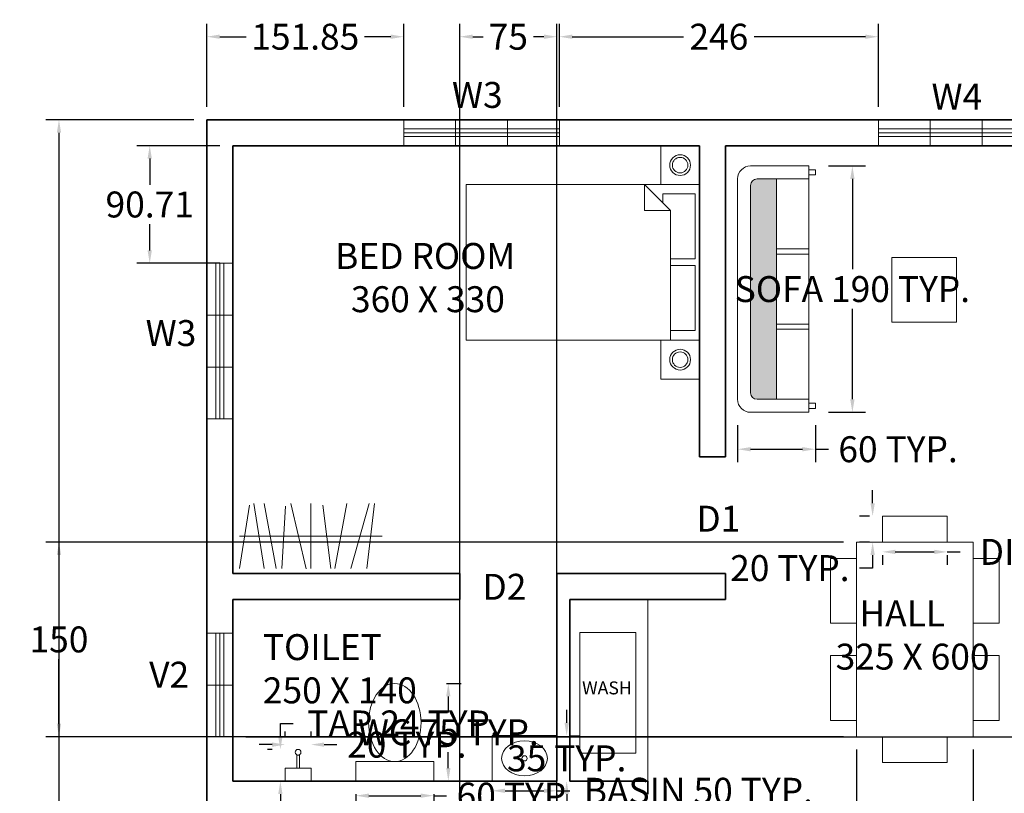
# Model space of a CAD drawing. Units: centimetres. Extents: x 543 to 2148, y 348 to 1642.
# Tile 2 of 4: x 543 to 1302, y 1046 to 1642. Entities that reach past the tile are written whole.
import ezdxf

# ---------------------------------------------------------------- set-up
doc = ezdxf.new("R2010")
doc.units = ezdxf.units.CM
doc.header["$MEASUREMENT"] = 0
for name, color, linetype, lineweight in [('A-ANNO-DIMS', 2, 'Continuous', 18), ('A-ANNO-TEXT', 7, 'Continuous', 18), ('A-AREA-IDEN', 7, 'Continuous', 25), ('A-FLOR-CASE', 8, 'Continuous', 20), ('A-FLOR-FIXT', 8, 'Continuous', 18), ('A-FURN', 8, 'Continuous', 18), ('A-FURN-PATT', 252, 'Continuous', 13), ('A-GLAZ', 4, 'Continuous', 18), ('A-WALL', 7, 'Continuous', 35)]:
    doc.layers.add(name, color=color, linetype=linetype, lineweight=lineweight)
doc.styles.get("Standard").update_dxf_attribs({"font": 'arial.ttf'})
doc.dimstyles.get("Standard").update_dxf_attribs({"dimtxt": 20, "dimasz": 10, "dimexe": 10, "dimexo": 10, "dimgap": 5, "dimtad": 0, "dimtih": 1, "dimtoh": 1, "dimdec": 0, "dimzin": 0, "dimdsep": 46, "dimtxsty": 'Standard', "dimcen": 5, "dimadec": 0, "dimazin": 0, "dimtfac": 1, "dimtdec": 0, "dimtofl": 0, "dimtmove": 0, "dimatfit": 3, "dimfxl": 1, "dimtolj": 1, "dimtzin": 0, "dimarcsym": 0})

# ---------------------------------------------------------------- blocks, each defined once
blk = doc.blocks.new('BED-DOUBLE')
for p, q in [((42.36, 150), (22.36, 130)), ((42.36, 130), (42.36, 150)), ((22.36, 130), (22.36, 30)), ((22.36, 130), (42.36, 130)), ((3.32, 102.87), (3.32, 92.87)), ((3.32, 92.87), (22.36, 92.87)), ((3.32, 77.49), (3.32, 87.49)), ((3.32, 87.49), (22.36, 87.49))]:
    blk.add_line(p, q)
for points in [[(0, 150), (30, 150), (30, 180), (0, 180)], [(180, 150), (180, 30), (0, 30), (0, 150)], [(0, 0), (30, 0), (30, 30), (0, 30)]]:
    blk.add_lwpolyline(points, close=True)
for points in [[(3.32, 102.87), (3.32, 142.87), (28.32, 142.87), (28.32, 135.96)], [(22.36, 37.49), (3.32, 37.49), (3.32, 77.49)]]:
    blk.add_lwpolyline(points)
for centre, radius in [((15, 165), 8), ((15, 165), 6), ((15, 15), 8), ((15, 15), 6)]:
    blk.add_circle(centre, radius)
blk = doc.blocks.new('SOFA-3SEAT')
for p, q in [((10, 190), (55, 190)), ((55, 190), (55, 125.56)), ((55, 190), (55, 187)), ((55, 187), (60, 187)), ((60, 183), (55, 183)), ((60, 187), (60, 183)), ((0, 125.56), (0, 180)), ((10, 125.56), (10, 175)), ((15, 180), (55, 180)), ((30, 125.56), (30, 180)), ((0, 10), (0, 125.56)), ((10, 15), (10, 125.56)), ((55, 126), (30, 126)), ((30, 10), (30, 125.56)), ((55, 122), (30, 122)), ((55, 125.56), (55, 0)), ((55, 68), (30, 68)), ((55, 64), (30, 64)), ((55, 10), (15, 10)), ((55, 0), (10, 0)), ((60, 7), (55, 7)), ((55, 0), (55, 3)), ((55, 3), (60, 3)), ((60, 3), (60, 7))]:
    blk.add_line(p, q)
for centre, radius, start, end in [((10, 180), 10, 90, 180), ((15, 175), 5, 90, 180), ((10, 10), 10, 180, 270), ((15, 15), 5, 180, 270)]:
    blk.add_arc(centre, radius, start, end)
blk = doc.blocks.new('WARDROBE-RAIL')
for p, q in [((0, 0.31), (7.78, 49.18)), ((11.01, 50.31), (19.09, 0.31)), ((19.09, 50.31), (28.16, 0.3)), ((32.55, 0.31), (35.53, 48.25)), ((39.55, 50.31), (51.34, 0)), ((55, 0.31), (55, 50.31)), ((64.34, 49.01), (70.51, 0.27)), ((73.48, 0.31), (82.64, 50.31)), ((99.87, 50.31), (85.87, 0.31)), ((98.25, 0.31), (103.96, 50.31)), ((0, 25.31), (110, 25.31))]:
    blk.add_line(p, q)
blk = doc.blocks.new('WIN-1200')
for p, q in [((40, 20), (40, 0)), ((80, 20), (80, 0)), ((0, 13), (120, 13)), ((0, 10), (120, 10)), ((0, 7), (120, 7))]:
    blk.add_line(p, q)
blk.add_lwpolyline([(0, 20), (120, 20), (120, 0), (0, 0)], close=True)
blk = doc.blocks.new('VENT-800')
for p, q in [((7, 80), (7, 0)), ((10, 80), (10, 0)), ((13, 80), (13, 0)), ((20, 40), (0, 40)), ((20, 0), (0, 0))]:
    blk.add_line(p, q)
blk.add_lwpolyline([(0, 0), (0, 80), (20, 80), (20, 0)])
blk = doc.blocks.new('WC')
blk.add_lwpolyline([(60, 0), (0, 0), (0, 15), (60, 15)], close=True)
blk.add_ellipse((30, 45.11), major_axis=(0, 30.11), ratio=0.671585)
blk = doc.blocks.new('WASHBASIN')
blk.add_lwpolyline([(50, 0), (0, 0), (0, 35), (50, 35)], close=True)
blk.add_circle((25, 17.5), 2)
blk.add_ellipse((25, 17.5), major_axis=(17.65, 0), ratio=0.767259)
blk = doc.blocks.new('WALL-TAP')
for p, q in [((9, 10), (9, 20)), ((9, 20), (11, 20)), ((11, 10), (11, 20))]:
    blk.add_line(p, q)
blk.add_lwpolyline([(0, 0), (20, 0), (20, 10), (0, 10)], close=True)
blk.add_circle((10, 22.21), 2.21)
blk = doc.blocks.new('CHAIR-DINING')
blk.add_lwpolyline([(0, 50), (0, 0), (20, 0), (20, 50)], close=True)
blk = doc.blocks.new('TABLE-SIDE')
blk.add_lwpolyline([(0, 50), (50, 50), (50, 0), (0, 0)], close=True)
blk = doc.blocks.new('*D15')
at = {"layer": 'A-ANNO-DIMS', "color": 0, "lineweight": -2, "transparency": 16777216}
for p, q in [((1218.09, 1231.81), (1248.09, 1231.81)), ((1258.09, 1231.81), (1268.09, 1231.81)), ((1208.09, 1229.31), (1208.09, 1221.81)), ((1258.09, 1229.31), (1258.09, 1221.81))]:
    blk.add_line(p, q, dxfattribs=at)
at = {"layer": 'A-ANNO-DIMS', "color": 0, "transparency": 16777216}
for points in [[(1218.09, 1233.48), (1218.09, 1230.15), (1208.09, 1231.81)], [(1248.09, 1233.48), (1248.09, 1230.15), (1258.09, 1231.81)]]:
    blk.add_solid(points, dxfattribs=at)
at = {"layer": 'Defpoints', "color": 0, "transparency": 16777216}
for p in [(1208.09, 1239.31), (1258.09, 1239.31), (1258.09, 1231.81)]:
    blk.add_point(p, dxfattribs=at)
at = {"layer": 'A-ANNO-DIMS', "color": 0, "transparency": 16777216, "insert": (1421.4, 1231.81), "char_height": 20, "attachment_point": 5}
blk.add_mtext('\\A1;DINING CHAIR 50 TYP.', dxfattribs=at)
blk = doc.blocks.new('*D16')
at = {"layer": 'A-ANNO-DIMS', "color": 0, "lineweight": -2, "transparency": 16777216}
for p, q in [((1200.59, 1269.31), (1200.59, 1279.31)), ((1198.09, 1259.31), (1190.59, 1259.31)), ((1198.09, 1239.31), (1190.59, 1239.31)), ((1200.59, 1229.31), (1200.59, 1219.31)), ((1200.59, 1219.31), (1190.59, 1219.31))]:
    blk.add_line(p, q, dxfattribs=at)
at = {"layer": 'A-ANNO-DIMS', "color": 0, "transparency": 16777216}
for points in [[(1198.93, 1269.31), (1202.26, 1269.31), (1200.59, 1259.31)], [(1198.93, 1229.31), (1202.26, 1229.31), (1200.59, 1239.31)]]:
    blk.add_solid(points, dxfattribs=at)
at = {"layer": 'Defpoints', "color": 0, "transparency": 16777216}
for p in [(1208.09, 1259.31), (1200.59, 1239.31), (1208.09, 1239.31)]:
    blk.add_point(p, dxfattribs=at)
at = {"layer": 'A-ANNO-DIMS', "color": 0, "transparency": 16777216, "insert": (1136.75, 1219.31), "char_height": 20, "attachment_point": 5}
blk.add_mtext('\\A1;20 TYP.', dxfattribs=at)
blk = doc.blocks.new('*D23')
at = {"layer": 'A-ANNO-DIMS', "color": 0, "lineweight": -2, "transparency": 16777216}
for p, q in [((1166.48, 1529.5), (1194.98, 1529.5)), ((1184.98, 1519.5), (1184.98, 1449.85)), ((1184.98, 1349.5), (1184.98, 1419.16)), ((1166.48, 1339.5), (1194.98, 1339.5))]:
    blk.add_line(p, q, dxfattribs=at)
at = {"layer": 'A-ANNO-DIMS', "color": 0, "transparency": 16777216}
for points in [[(1183.31, 1519.5), (1186.65, 1519.5), (1184.98, 1529.5)], [(1183.31, 1349.5), (1186.65, 1349.5), (1184.98, 1339.5)]]:
    blk.add_solid(points, dxfattribs=at)
at = {"layer": 'Defpoints', "color": 0, "transparency": 16777216}
for p in [(1156.48, 1529.5), (1184.98, 1529.5), (1156.48, 1339.5)]:
    blk.add_point(p, dxfattribs=at)
at = {"layer": 'A-ANNO-DIMS', "color": 0, "transparency": 16777216, "insert": (1184.98, 1434.5), "char_height": 20, "attachment_point": 5}
blk.add_mtext('\\A1;SOFA 190 TYP.', dxfattribs=at)
blk = doc.blocks.new('*D24')
at = {"layer": 'A-ANNO-DIMS', "color": 0, "lineweight": -2, "transparency": 16777216}
for p, q in [((1096.48, 1329.5), (1096.48, 1301)), ((1156.48, 1329.5), (1156.48, 1301)), ((1106.48, 1311), (1146.48, 1311)), ((1156.48, 1311), (1166.48, 1311))]:
    blk.add_line(p, q, dxfattribs=at)
at = {"layer": 'A-ANNO-DIMS', "color": 0, "transparency": 16777216}
for points in [[(1106.48, 1312.67), (1106.48, 1309.34), (1096.48, 1311)], [(1146.48, 1312.67), (1146.48, 1309.34), (1156.48, 1311)]]:
    blk.add_solid(points, dxfattribs=at)
at = {"layer": 'Defpoints', "color": 0, "transparency": 16777216}
for p in [(1096.48, 1339.5), (1156.48, 1339.5), (1156.48, 1311)]:
    blk.add_point(p, dxfattribs=at)
at = {"layer": 'A-ANNO-DIMS', "color": 0, "transparency": 16777216, "insert": (1220.21, 1311), "char_height": 20, "attachment_point": 5}
blk.add_mtext('\\A1;60 TYP.', dxfattribs=at)
blk = doc.blocks.new('*D29')
at = {"layer": 'A-ANNO-DIMS', "color": 0, "lineweight": -2, "transparency": 16777216}
for p, q in [((872.08, 1130.32), (883.37, 1130.32)), ((873.37, 1120.32), (873.37, 1108.05)), ((873.37, 1065.09), (873.37, 1077.36)), ((872.08, 1055.09), (883.37, 1055.09))]:
    blk.add_line(p, q, dxfattribs=at)
at = {"layer": 'A-ANNO-DIMS', "color": 0, "transparency": 16777216}
for points in [[(871.7, 1120.32), (875.03, 1120.32), (873.37, 1130.32)], [(871.7, 1065.09), (875.03, 1065.09), (873.37, 1055.09)]]:
    blk.add_solid(points, dxfattribs=at)
at = {"layer": 'Defpoints', "color": 0, "transparency": 16777216}
for p in [(862.08, 1130.32), (873.37, 1130.32), (862.08, 1055.09)]:
    blk.add_point(p, dxfattribs=at)
at = {"layer": 'A-ANNO-DIMS', "color": 0, "transparency": 16777216, "insert": (873.37, 1092.7), "char_height": 20, "attachment_point": 5}
blk.add_mtext('\\A1;WC 75 TYP.', dxfattribs=at)
blk = doc.blocks.new('*D30')
at = {"layer": 'A-ANNO-DIMS', "color": 0, "lineweight": -2, "transparency": 16777216}
for p, q in [((802.08, 1045.09), (802.08, 1033.81)), ((812.08, 1043.81), (852.08, 1043.81)), ((862.08, 1045.09), (862.08, 1033.81)), ((862.08, 1043.81), (872.08, 1043.81))]:
    blk.add_line(p, q, dxfattribs=at)
at = {"layer": 'A-ANNO-DIMS', "color": 0, "transparency": 16777216}
for points in [[(812.08, 1045.47), (812.08, 1042.14), (802.08, 1043.81)], [(852.08, 1045.47), (852.08, 1042.14), (862.08, 1043.81)]]:
    blk.add_solid(points, dxfattribs=at)
at = {"layer": 'Defpoints', "color": 0, "transparency": 16777216}
for p in [(802.08, 1055.09), (862.08, 1055.09), (862.08, 1043.81)]:
    blk.add_point(p, dxfattribs=at)
at = {"layer": 'A-ANNO-DIMS', "color": 0, "transparency": 16777216, "insert": (925.81, 1043.81), "char_height": 20, "attachment_point": 5}
blk.add_mtext('\\A1;60 TYP.', dxfattribs=at)
blk = doc.blocks.new('*D31')
at = {"layer": 'A-ANNO-DIMS', "color": 0, "lineweight": -2, "transparency": 16777216}
for p, q in [((907.14, 1045.09), (907.14, 1037.59)), ((917.14, 1047.59), (947.14, 1047.59)), ((957.14, 1047.59), (967.14, 1047.59)), ((957.14, 1045.09), (957.14, 1037.59))]:
    blk.add_line(p, q, dxfattribs=at)
at = {"layer": 'A-ANNO-DIMS', "color": 0, "transparency": 16777216}
for points in [[(917.14, 1049.26), (917.14, 1045.93), (907.14, 1047.59)], [(947.14, 1049.26), (947.14, 1045.93), (957.14, 1047.59)]]:
    blk.add_solid(points, dxfattribs=at)
at = {"layer": 'Defpoints', "color": 0, "transparency": 16777216}
for p in [(907.14, 1055.09), (957.14, 1055.09), (957.14, 1047.59)]:
    blk.add_point(p, dxfattribs=at)
at = {"layer": 'A-ANNO-DIMS', "color": 0, "transparency": 16777216, "insert": (1066.18, 1047.59), "char_height": 20, "attachment_point": 5}
blk.add_mtext('\\A1;BASIN 50 TYP.', dxfattribs=at)
blk = doc.blocks.new('*D32')
at = {"layer": 'A-ANNO-DIMS', "color": 0, "lineweight": -2, "transparency": 16777216}
for p, q in [((964.64, 1100.09), (964.64, 1110.09)), ((967.14, 1090.09), (974.64, 1090.09)), ((967.14, 1055.09), (974.64, 1055.09)), ((964.64, 1045.09), (964.64, 1035.09))]:
    blk.add_line(p, q, dxfattribs=at)
at = {"layer": 'A-ANNO-DIMS', "color": 0, "transparency": 16777216}
for points in [[(962.97, 1100.09), (966.31, 1100.09), (964.64, 1090.09)], [(962.97, 1045.09), (966.31, 1045.09), (964.64, 1055.09)]]:
    blk.add_solid(points, dxfattribs=at)
at = {"layer": 'Defpoints', "color": 0, "transparency": 16777216}
for p in [(957.14, 1090.09), (964.64, 1090.09), (957.14, 1055.09)]:
    blk.add_point(p, dxfattribs=at)
at = {"layer": 'A-ANNO-DIMS', "color": 0, "transparency": 16777216, "insert": (964.64, 1072.59), "char_height": 20, "attachment_point": 5}
blk.add_mtext('\\A1;35 TYP.', dxfattribs=at)
blk = doc.blocks.new('*D33')
at = {"layer": 'A-ANNO-DIMS', "color": 0, "lineweight": -2, "transparency": 16777216}
for p, q in [((743.83, 1089.51), (743.83, 1099.51)), ((743.83, 1099.51), (753.83, 1099.51)), ((737.5, 1079.51), (733.83, 1079.51)), ((737.5, 1055.09), (733.83, 1055.09)), ((743.83, 1045.09), (743.83, 1035.09))]:
    blk.add_line(p, q, dxfattribs=at)
at = {"layer": 'A-ANNO-DIMS', "color": 0, "transparency": 16777216}
for points in [[(742.17, 1089.51), (745.5, 1089.51), (743.83, 1079.51)], [(742.17, 1045.09), (745.5, 1045.09), (743.83, 1055.09)]]:
    blk.add_solid(points, dxfattribs=at)
at = {"layer": 'Defpoints', "color": 0, "transparency": 16777216}
for p in [(743.83, 1079.51), (747.5, 1079.51), (747.5, 1055.09)]:
    blk.add_point(p, dxfattribs=at)
at = {"layer": 'A-ANNO-DIMS', "color": 0, "transparency": 16777216, "insert": (838.81, 1099.51), "char_height": 20, "attachment_point": 5}
blk.add_mtext('\\A1;TAP 24 TYP.', dxfattribs=at)
blk = doc.blocks.new('*D34')
at = {"layer": 'A-ANNO-DIMS', "color": 0, "lineweight": -2, "transparency": 16777216}
for p, q in [((747.5, 1089.51), (747.5, 1093.18)), ((767.5, 1089.51), (767.5, 1093.18)), ((737.5, 1083.18), (727.5, 1083.18)), ((777.5, 1083.18), (787.5, 1083.18))]:
    blk.add_line(p, q, dxfattribs=at)
at = {"layer": 'A-ANNO-DIMS', "color": 0, "transparency": 16777216}
for points in [[(737.5, 1084.84), (737.5, 1081.51), (747.5, 1083.18)], [(777.5, 1084.84), (777.5, 1081.51), (767.5, 1083.18)]]:
    blk.add_solid(points, dxfattribs=at)
at = {"layer": 'Defpoints', "color": 0, "transparency": 16777216}
for p in [(747.5, 1079.51), (767.5, 1083.18), (767.5, 1079.51)]:
    blk.add_point(p, dxfattribs=at)
at = {"layer": 'A-ANNO-DIMS', "color": 0, "transparency": 16777216, "insert": (841.34, 1083.18), "char_height": 20, "attachment_point": 5}
blk.add_mtext('\\A1;20 TYP.', dxfattribs=at)
blk = doc.blocks.new('*D44')
at = {"layer": 'A-ANNO-DIMS', "color": 0, "lineweight": -2, "transparency": 16777216}
for p, q in [((882.14, 895.09), (882.14, 1639.14)), ((957.14, 895.09), (957.14, 1639.14)), ((892.14, 1629.14), (900.32, 1629.14)), ((947.14, 1629.14), (938.96, 1629.14))]:
    blk.add_line(p, q, dxfattribs=at)
at = {"layer": 'A-ANNO-DIMS', "color": 0, "transparency": 16777216}
for points in [[(892.14, 1630.81), (892.14, 1627.48), (882.14, 1629.14)], [(947.14, 1630.81), (947.14, 1627.48), (957.14, 1629.14)]]:
    blk.add_solid(points, dxfattribs=at)
at = {"layer": 'Defpoints', "color": 0, "transparency": 16777216}
for p in [(957.14, 1629.14), (882.14, 885.09), (957.14, 885.09)]:
    blk.add_point(p, dxfattribs=at)
at = {"layer": 'A-ANNO-DIMS', "color": 0, "transparency": 16777216, "insert": (919.64, 1629.14), "char_height": 20, "attachment_point": 5}
blk.add_mtext('\\A1;75', dxfattribs=at)
blk = doc.blocks.new('*D48')
at = {"layer": 'A-ANNO-DIMS', "color": 0, "lineweight": -2, "transparency": 16777216}
for p, q in [((687.14, 1575.09), (687.14, 1639.14)), ((838.99, 1575.09), (838.99, 1639.14)), ((697.14, 1629.14), (717.42, 1629.14)), ((828.99, 1629.14), (808.71, 1629.14))]:
    blk.add_line(p, q, dxfattribs=at)
at = {"layer": 'A-ANNO-DIMS', "color": 0, "transparency": 16777216}
for points in [[(697.14, 1630.81), (697.14, 1627.48), (687.14, 1629.14)], [(828.99, 1630.81), (828.99, 1627.48), (838.99, 1629.14)]]:
    blk.add_solid(points, dxfattribs=at)
at = {"layer": 'Defpoints', "color": 0, "transparency": 16777216}
for p in [(838.99, 1629.14), (687.14, 1565.09), (838.99, 1565.09)]:
    blk.add_point(p, dxfattribs=at)
at = {"layer": 'A-ANNO-DIMS', "color": 0, "transparency": 16777216, "insert": (763.06, 1629.14), "char_height": 20, "attachment_point": 5}
blk.add_mtext('\\A1;151.85', dxfattribs=at)
blk = doc.blocks.new('*D49')
at = {"layer": 'A-ANNO-DIMS', "color": 0, "lineweight": -2, "transparency": 16777216}
for p, q in [((958.99, 1575.09), (958.99, 1639.14)), ((1205.01, 1575.09), (1205.01, 1639.14)), ((968.99, 1629.14), (1054.74, 1629.14)), ((1195.01, 1629.14), (1109.25, 1629.14))]:
    blk.add_line(p, q, dxfattribs=at)
at = {"layer": 'A-ANNO-DIMS', "color": 0, "transparency": 16777216}
for points in [[(968.99, 1630.81), (968.99, 1627.48), (958.99, 1629.14)], [(1195.01, 1630.81), (1195.01, 1627.48), (1205.01, 1629.14)]]:
    blk.add_solid(points, dxfattribs=at)
at = {"layer": 'Defpoints', "color": 0, "transparency": 16777216}
for p in [(1205.01, 1629.14), (958.99, 1565.09), (1205.01, 1565.09)]:
    blk.add_point(p, dxfattribs=at)
at = {"layer": 'A-ANNO-DIMS', "color": 0, "transparency": 16777216, "insert": (1082, 1629.14), "char_height": 20, "attachment_point": 5}
blk.add_mtext('\\A1;246', dxfattribs=at)
blk = doc.blocks.new('*D59')
at = {"layer": 'A-ANNO-DIMS', "color": 0, "lineweight": -2, "transparency": 16777216}
for p, q in [((717.14, 1089.08), (1916.19, 1089.08)), ((1906.19, 1079.08), (1906.19, 1065.14)), ((1906.19, 1020.76), (1906.19, 1034.7)), ((717.14, 1010.76), (1916.19, 1010.76))]:
    blk.add_line(p, q, dxfattribs=at)
at = {"layer": 'A-ANNO-DIMS', "color": 0, "transparency": 16777216}
for points in [[(1904.52, 1079.08), (1907.86, 1079.08), (1906.19, 1089.08)], [(1904.52, 1020.76), (1907.86, 1020.76), (1906.19, 1010.76)]]:
    blk.add_solid(points, dxfattribs=at)
at = {"layer": 'Defpoints', "color": 0, "transparency": 16777216}
for p in [(707.14, 1089.08), (1906.19, 1089.08), (707.14, 1010.76)]:
    blk.add_point(p, dxfattribs=at)
at = {"layer": 'A-ANNO-DIMS', "color": 0, "transparency": 16777216, "insert": (1906.19, 1049.92), "char_height": 20, "attachment_point": 5}
blk.add_mtext('\\A1;78.33', dxfattribs=at)
blk = doc.blocks.new('*D60')
at = {"layer": 'A-ANNO-DIMS', "color": 0, "lineweight": -2, "transparency": 16777216}
for p, q in [((697.14, 1545.09), (633.09, 1545.09)), ((643.09, 1535.09), (643.09, 1514.95)), ((643.09, 1464.38), (643.09, 1484.52)), ((697.14, 1454.38), (633.09, 1454.38))]:
    blk.add_line(p, q, dxfattribs=at)
at = {"layer": 'A-ANNO-DIMS', "color": 0, "transparency": 16777216}
for points in [[(641.42, 1535.09), (644.76, 1535.09), (643.09, 1545.09)], [(641.42, 1464.38), (644.76, 1464.38), (643.09, 1454.38)]]:
    blk.add_solid(points, dxfattribs=at)
at = {"layer": 'Defpoints', "color": 0, "transparency": 16777216}
for p in [(643.09, 1545.09), (707.14, 1545.09), (707.14, 1454.38)]:
    blk.add_point(p, dxfattribs=at)
at = {"layer": 'A-ANNO-DIMS', "color": 0, "transparency": 16777216, "insert": (643.09, 1499.74), "char_height": 20, "attachment_point": 5}
blk.add_mtext('\\A1;90.71', dxfattribs=at)
blk = doc.blocks.new('*D64')
at = {"layer": 'A-ANNO-DIMS', "color": 0, "lineweight": -2, "transparency": 16777216}
for p, q in [((1188.09, 1079.31), (1188.09, 351.04)), ((1278.09, 1079.31), (1278.09, 351.04)), ((1198.09, 361.04), (1213.8, 361.04)), ((1268.09, 361.04), (1252.38, 361.04))]:
    blk.add_line(p, q, dxfattribs=at)
at = {"layer": 'A-ANNO-DIMS', "color": 0, "transparency": 16777216}
for points in [[(1198.09, 362.71), (1198.09, 359.38), (1188.09, 361.04)], [(1268.09, 362.71), (1268.09, 359.38), (1278.09, 361.04)]]:
    blk.add_solid(points, dxfattribs=at)
at = {"layer": 'Defpoints', "color": 0, "transparency": 16777216}
for p in [(1188.09, 1089.31), (1278.09, 1089.31), (1278.09, 361.04)]:
    blk.add_point(p, dxfattribs=at)
at = {"layer": 'A-ANNO-DIMS', "color": 0, "transparency": 16777216, "insert": (1233.09, 361.04), "char_height": 20, "attachment_point": 5}
blk.add_mtext('\\A1;90', dxfattribs=at)
blk = doc.blocks.new('*D65')
at = {"layer": 'A-ANNO-DIMS', "color": 0, "lineweight": -2, "transparency": 16777216}
for p, q in [((1178.09, 1239.31), (563.09, 1239.31)), ((573.09, 1229.31), (573.09, 1179.52)), ((573.09, 1099.31), (573.09, 1149.1)), ((1178.09, 1089.31), (563.09, 1089.31))]:
    blk.add_line(p, q, dxfattribs=at)
at = {"layer": 'A-ANNO-DIMS', "color": 0, "transparency": 16777216}
for points in [[(571.42, 1229.31), (574.76, 1229.31), (573.09, 1239.31)], [(571.42, 1099.31), (574.76, 1099.31), (573.09, 1089.31)]]:
    blk.add_solid(points, dxfattribs=at)
at = {"layer": 'Defpoints', "color": 0, "transparency": 16777216}
for p in [(1188.09, 1239.31), (573.09, 1089.31), (1188.09, 1089.31)]:
    blk.add_point(p, dxfattribs=at)
at = {"layer": 'A-ANNO-DIMS', "color": 0, "transparency": 16777216, "insert": (573.09, 1164.31), "char_height": 20, "attachment_point": 5}
blk.add_mtext('\\A1;150', dxfattribs=at)
blk = doc.blocks.new('*D67')
at = {"layer": 'A-ANNO-DIMS', "color": 0, "lineweight": -2, "transparency": 16777216}
for p, q in [((677.14, 1565.09), (563.09, 1565.09)), ((573.09, 1555.09), (573.09, 1010.3)), ((573.09, 435.09), (573.09, 979.88)), ((627.14, 425.09), (563.09, 425.09))]:
    blk.add_line(p, q, dxfattribs=at)
at = {"layer": 'A-ANNO-DIMS', "color": 0, "transparency": 16777216}
for points in [[(571.42, 1555.09), (574.76, 1555.09), (573.09, 1565.09)], [(571.42, 435.09), (574.76, 435.09), (573.09, 425.09)]]:
    blk.add_solid(points, dxfattribs=at)
at = {"layer": 'Defpoints', "color": 0, "transparency": 16777216}
for p in [(573.09, 1565.09), (687.14, 1565.09), (637.14, 425.09)]:
    blk.add_point(p, dxfattribs=at)
at = {"layer": 'A-ANNO-DIMS', "color": 0, "transparency": 16777216, "insert": (573.09, 995.09), "char_height": 20, "attachment_point": 5}
blk.add_mtext('\\A1;1140', dxfattribs=at)
blk = doc.blocks.new('*D68')
at = {"layer": 'A-ANNO-DIMS', "color": 0, "lineweight": -2, "transparency": 16777216}
for p, q in [((1842.14, 1185.09), (1842.14, 351.04)), ((637.14, 415.09), (637.14, 351.04)), ((647.14, 361.04), (1205.64, 361.04)), ((1832.14, 361.04), (1273.64, 361.04))]:
    blk.add_line(p, q, dxfattribs=at)
at = {"layer": 'A-ANNO-DIMS', "color": 0, "transparency": 16777216}
for points in [[(647.14, 362.71), (647.14, 359.38), (637.14, 361.04)], [(1832.14, 362.71), (1832.14, 359.38), (1842.14, 361.04)]]:
    blk.add_solid(points, dxfattribs=at)
at = {"layer": 'Defpoints', "color": 0, "transparency": 16777216}
for p in [(1842.14, 1195.09), (637.14, 425.09), (1842.14, 361.04)]:
    blk.add_point(p, dxfattribs=at)
at = {"layer": 'A-ANNO-DIMS', "color": 0, "transparency": 16777216, "insert": (1239.64, 361.04), "char_height": 20, "attachment_point": 5}
blk.add_mtext('\\A1;1205', dxfattribs=at)

msp = doc.modelspace()

# ---------------------------------------------------------------- hatches: boundary and pattern name
at = {"layer": 'A-FURN-PATT'}
h = msp.add_hatch(dxfattribs=at)
h.set_pattern_fill('CROSS', color=256, scale=25)
h.paths.add_polyline_path([(1290.635, 688.693), (1175.07, 688.693), (1120.635, 688.693), (1120.635, 673.693, 0.4142136), (1125.635, 668.693), (1175.07, 668.693), (1285.635, 668.693, 0.4142136), (1290.635, 673.693)])
h.paths.add_polyline_path([(1105.412, 856.024), (1105.412, 910.459), (1090.412, 910.459, 0.4142136), (1085.412, 905.459), (1085.412, 856.024), (1085.412, 745.459, 0.4142136), (1090.412, 740.459), (1105.412, 740.459)])
h.paths.add_polyline_path([(1126.48, 1465.069), (1126.48, 1519.504), (1111.48, 1519.504, 0.4142136), (1106.48, 1514.504), (1106.48, 1465.069), (1106.48, 1354.504, 0.4142136), (1111.48, 1349.504), (1126.48, 1349.504)])

# ---------------------------------------------------------------- linework, layer by layer
at = {"layer": 'A-FLOR-CASE'}
msp.add_line((1027.141, 1055.092), (1027.141, 1195.092), dxfattribs=at)
at = {"layer": 'A-FLOR-FIXT'}
msp.add_lwpolyline([(974.732, 1169.562), (1017.895, 1169.562), (1017.895, 1076.701), (974.732, 1076.701)], close=True, dxfattribs=at)
at = {"layer": 'A-FURN'}
msp.add_lwpolyline([(1278.094, 1239.313), (1278.094, 1089.313), (1188.094, 1089.313), (1188.094, 1239.313)], close=True, dxfattribs=at)
at = {"layer": 'A-WALL'}
for p, q in [((687.141, 1565.092), (687.141, 885.092)), ((1412.141, 1565.092), (687.141, 1565.092)), ((707.141, 1545.092), (1067.141, 1545.092)), ((707.141, 1215.092), (707.141, 1545.092)), ((1067.141, 1545.092), (1067.141, 1305.092)), ((1087.141, 1545.092), (1412.141, 1545.092)), ((1087.141, 1305.092), (1087.141, 1545.092)), ((1067.141, 1305.092), (1087.141, 1305.092)), ((882.141, 1215.092), (707.141, 1215.092)), ((882.141, 1215.092), (882.141, 1195.092)), ((1067.141, 1215.092), (957.141, 1215.092)), ((957.141, 1215.092), (957.141, 1195.092)), ((1067.141, 1215.092), (1087.141, 1215.092)), ((1087.141, 1195.092), (1087.141, 1215.092)), ((707.141, 1195.092), (882.141, 1195.092)), ((707.141, 1055.092), (707.141, 1195.092)), ((957.141, 1195.092), (957.141, 1055.092)), ((967.141, 1195.092), (1067.141, 1195.092)), ((967.141, 1055.092), (967.141, 1195.092)), ((1067.141, 1195.092), (1087.141, 1195.092)), ((957.141, 1055.092), (707.141, 1055.092)), ((967.141, 1055.092), (1027.141, 1055.092)), ((1027.141, 1055.092), (1027.141, 1045.092))]:
    msp.add_line(p, q, dxfattribs=at)

# ---------------------------------------------------------------- block references
at = {"layer": 'A-FLOR-CASE'}
msp.add_blockref('WARDROBE-RAIL', (712.346, 1218.721), dxfattribs=at)
at = {"layer": 'A-FLOR-FIXT'}
for name, p in [('WC', (802.082, 1055.092)), ('WASHBASIN', (907.141, 1055.092)), ('WALL-TAP', (747.497, 1055.092))]:
    msp.add_blockref(name, p, dxfattribs=at)
at = {"layer": 'A-FURN', "extrusion": (0, 0, -1), "zscale": -1}
msp.add_blockref('BED-DOUBLE', (-1067.141, 1365.091), dxfattribs=at)
at = {"layer": 'A-FURN'}
for name, p in [('SOFA-3SEAT', (1096.48, 1339.504)), ('TABLE-SIDE', (1215.296, 1408.865)), ('CHAIR-DINING', (1168.094, 1176.813)), ('CHAIR-DINING', (1278.094, 1176.813)), ('CHAIR-DINING', (1168.094, 1101.813)), ('CHAIR-DINING', (1278.094, 1101.813))]:
    msp.add_blockref(name, p, dxfattribs=at)
at = {"layer": 'A-FURN', "rotation": 270.0000000000005}
for p in [(1208.094, 1259.313), (1208.094, 1089.313)]:
    msp.add_blockref('CHAIR-DINING', p, dxfattribs=at)
at = {"layer": 'A-GLAZ'}
for name, p in [('WIN-1200', (838.987, 1545.092)), ('WIN-1200', (1205.005, 1545.092)), ('VENT-800', (687.141, 1089.083))]:
    msp.add_blockref(name, p, dxfattribs=at)
at = {"layer": 'A-GLAZ', "rotation": 270.0000000000001}
msp.add_blockref('WIN-1200', (687.141, 1454.38), dxfattribs=at)

# ---------------------------------------------------------------- texts
at = {"layer": 'A-ANNO-TEXT', "char_height": 20, "attachment_point": 1}
for s, insert in [('W3', (876.177, 1594.247)), ('W4', (1246, 1592.989)), ('W3', (639.93, 1410.606)), ('D1', (1064.656, 1267.421)), ('D2', (899.667, 1214.899)), ('V2', (642.667, 1147.103))]:
    msp.add_mtext_dynamic_manual_height_columns(s, width=246.06417, gutter_width=1, heights=[0], dxfattribs=dict(at, insert=insert))
at = {"layer": 'A-AREA-IDEN', "attachment_point": 1}
for s, insert, char_height in [('BED ROOM\\P  360 X 330', (786.059, 1470.035), 20), ('      HALL\\P   325 X 600', (1153.722, 1194.377), 20), ('TOILET\\P250 X 140', (730.333, 1168.371), 20), ('WASH', (976.531, 1131.936), 10)]:
    msp.add_mtext_dynamic_manual_height_columns(s, width=246.06417, gutter_width=1, heights=[0], dxfattribs=dict(at, insert=insert, char_height=char_height))

# ---------------------------------------------------------------- dimensions: what is measured, and where the dimension line sits
at = {"layer": 'A-ANNO-DIMS'}
for base, p1, p2, override, picture, middle in [((838.987, 1629.142), (687.141, 1565.092), (838.987, 1565.092), {"dimdec": 2, "dimlfac": 1, "dimrnd": 0, "dimzin": 0, "dimdsep": 46, "dimlunit": 2}, '*D48', (763.064, 1629.142)), ((957.141, 1629.142), (882.141, 885.092), (957.141, 885.092), {"dimdec": 0, "dimlfac": 1, "dimrnd": 0, "dimzin": 0, "dimdsep": 46, "dimlunit": 2}, '*D44', (919.641, 1629.142)), ((1205.005, 1629.142), (958.987, 1565.092), (1205.005, 1565.092), {"dimdec": 0, "dimlfac": 1, "dimrnd": 0, "dimzin": 0, "dimdsep": 46, "dimlunit": 2}, '*D49', (1081.996, 1629.142)), ((1842.141, 361.042), (637.141, 425.092), (1842.141, 1195.092), {"dimdec": 0, "dimlfac": 1, "dimrnd": 0, "dimzin": 0, "dimdsep": 46, "dimlunit": 2}, '*D68', (1239.641, 361.042)), ((1278.094, 361.042), (1188.094, 1089.313), (1278.094, 1089.313), {"dimdec": 0, "dimlfac": 1, "dimrnd": 0, "dimzin": 0, "dimdsep": 46, "dimlunit": 2}, '*D64', (1233.094, 361.042))]:
    dim = msp.add_linear_dim(base=base, p1=p1, p2=p2, dimstyle='Standard', override=override, dxfattribs=at)
    dim.commit()
    dim.dimension.update_dxf_attribs({"geometry": picture, "text_midpoint": middle})
for base, p1, p2, override, picture, middle in [((573.091, 1565.092), (637.141, 425.092), (687.141, 1565.092), {"dimdec": 0, "dimlfac": 1, "dimrnd": 0, "dimzin": 0, "dimdsep": 46, "dimlunit": 2}, '*D67', (573.091, 995.092)), ((643.091, 1545.092), (707.141, 1454.38), (707.141, 1545.092), {"dimdec": 2, "dimlfac": 1, "dimrnd": 0, "dimzin": 0, "dimdsep": 46, "dimlunit": 2}, '*D60', (643.091, 1499.736)), ((573.091, 1089.313), (1188.094, 1239.313), (1188.094, 1089.313), {"dimdec": 0, "dimlfac": 1, "dimrnd": 0, "dimzin": 0, "dimdsep": 46, "dimlunit": 2}, '*D65', (573.091, 1164.313)), ((1906.1909, 1089.0833), (707.1409, 1010.7581), (707.1409, 1089.0833), {"dimdec": 2, "dimlfac": 1, "dimrnd": 0, "dimzin": 0, "dimdsep": 46, "dimlunit": 2}, '*D59', (1906.1909, 1049.9207))]:
    dim = msp.add_linear_dim(base=base, p1=p1, p2=p2, angle=90, dimstyle='Standard', override=override, dxfattribs=at)
    dim.commit()
    dim.dimension.update_dxf_attribs({"geometry": picture, "text_midpoint": middle})
for base, p1, p2, angle, text, picture, middle in [((1184.98, 1529.504), (1156.48, 1339.504), (1156.48, 1529.504), 90, 'SOFA <> TYP.', '*D23', (1184.98, 1434.504)), ((1258.094, 1231.813), (1208.094, 1239.313), (1258.094, 1239.313), 0, 'DINING CHAIR <> TYP.', '*D15', (1421.396, 1231.813)), ((1200.594, 1239.313), (1208.094, 1259.313), (1208.094, 1239.313), 270, '<> TYP.', '*D16', (1136.747, 1219.313)), ((743.834, 1079.513), (747.497, 1055.092), (747.497, 1079.513), 90, 'TAP <> TYP.', '*D33', (838.814, 1099.513)), ((873.366, 1130.318), (862.082, 1055.092), (862.082, 1130.318), 90, 'WC <> TYP.', '*D29', (873.366, 1092.705)), ((964.641, 1090.092), (957.141, 1055.092), (957.141, 1090.092), 90, '<> TYP.', '*D32', (964.641, 1072.592))]:
    dim = msp.add_linear_dim(base=base, p1=p1, p2=p2, angle=angle, text=text, dimstyle='Standard', override={"dimdec": 0, "dimlfac": 1, "dimrnd": 0, "dimzin": 0, "dimdsep": 46, "dimlunit": 2}, dxfattribs=at)
    dim.commit()
    dim.dimension.update_dxf_attribs({"geometry": picture, "text_midpoint": middle})
for base, p1, p2, text, picture, middle in [((1156.48, 1311.004), (1096.48, 1339.504), (1156.48, 1339.504), '<> TYP.', '*D24', (1220.211, 1311.004)), ((767.497, 1083.176), (747.497, 1079.513), (767.497, 1079.513), '<> TYP.', '*D34', (841.345, 1083.176)), ((957.141, 1047.592), (907.141, 1055.092), (957.141, 1055.092), 'BASIN <> TYP.', '*D31', (1066.179, 1047.592)), ((862.082, 1043.808), (802.082, 1055.092), (862.082, 1055.092), '<> TYP.', '*D30', (925.813, 1043.808))]:
    dim = msp.add_linear_dim(base=base, p1=p1, p2=p2, text=text, dimstyle='Standard', override={"dimdec": 0, "dimlfac": 1, "dimrnd": 0, "dimzin": 0, "dimdsep": 46, "dimlunit": 2}, dxfattribs=at)
    dim.commit()
    dim.dimension.update_dxf_attribs({"geometry": picture, "text_midpoint": middle})

doc.saveas('drawing.dxf')
